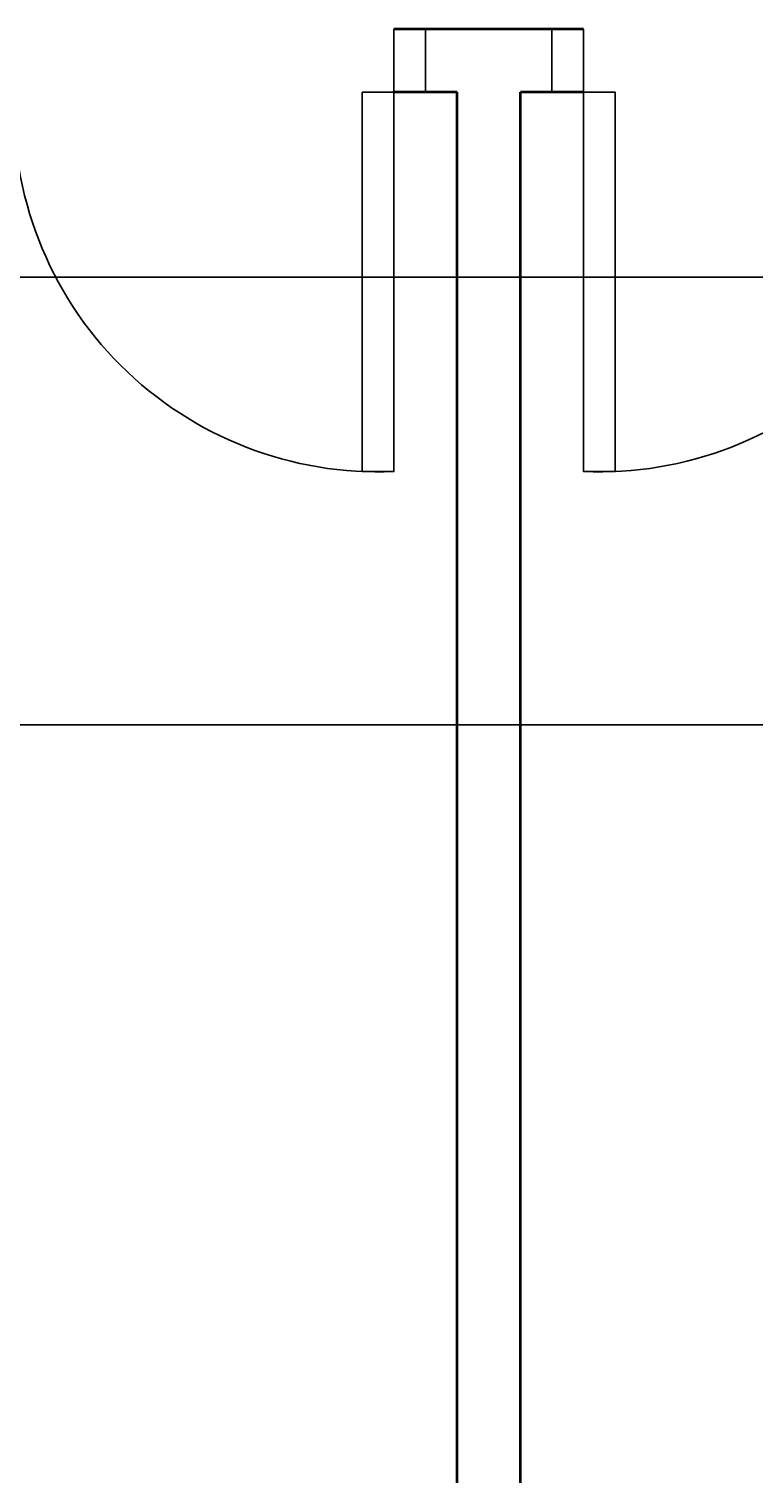
# Model space of a CAD drawing. Units: inches. Extents: x 4159 to 4826, y 299 to 1026.
# Tile 32 of 37: x 4617 to 4685, y 401 to 539. Entities that reach past the tile are written whole.
import ezdxf

# ---------------------------------------------------------------- set-up
doc = ezdxf.new("R2010")
doc.units = ezdxf.units.IN
for name, color, linetype, lineweight in [('A-ANNO-DIMS', 2, 'Continuous', 18), ('A-DOOR', 4, 'Continuous', 25), ('A-WALL', 7, 'Continuous', 35)]:
    doc.layers.add(name, color=color, linetype=linetype, lineweight=lineweight)
doc.styles.get("Standard").update_dxf_attribs({"font": 'arial.ttf'})
doc.dimstyles.get("Standard").update_dxf_attribs({"dimtxt": 0.18, "dimasz": 0.18, "dimexe": 0.18, "dimexo": 0.0625, "dimgap": 0.09, "dimtad": 0, "dimtih": 1, "dimtoh": 1, "dimdec": 4, "dimzin": 0, "dimdsep": 46, "dimtxsty": 'Standard', "dimcen": 0.09, "dimadec": 0, "dimazin": 0, "dimtfac": 1, "dimtdec": 4, "dimtofl": 0, "dimtmove": 0, "dimatfit": 3, "dimfxl": 1, "dimtolj": 1, "dimtzin": 0, "dimarcsym": 0})

# ---------------------------------------------------------------- blocks, each defined once
blk = doc.blocks.new('DOOR-SWING-36IN')
blk.add_lwpolyline([(0, 0), (-3, 0), (-3, 36), (0, 36)], close=True)
blk.add_arc((-1.5, 1.5), 34.53, 87.5104, 182.4896)
blk = doc.blocks.new('DOOR-FRAME-36IN')
for p, q in [((0, 6), (0, 0)), ((3, 6), (3, 0)), ((39, 6), (39, 0)), ((42, 6), (42, 0))]:
    blk.add_line(p, q)
blk = doc.blocks.new('*D54')
at = {"layer": 'A-ANNO-DIMS', "color": 0, "lineweight": -2, "transparency": 16777216}
for p, q in [((4501.37, 515.71), (4825.74, 515.71)), ((4825.56, 515.53), (4825.56, 494.64)), ((4825.56, 473.38), (4825.56, 494.27)), ((4541.95, 473.2), (4825.74, 473.2))]:
    blk.add_line(p, q, dxfattribs=at)
at = {"layer": 'A-ANNO-DIMS', "color": 0, "transparency": 16777216}
for points in [[(4825.53, 515.53), (4825.59, 515.53), (4825.56, 515.71)], [(4825.53, 473.38), (4825.59, 473.38), (4825.56, 473.2)]]:
    blk.add_solid(points, dxfattribs=at)
at = {"layer": 'Defpoints', "color": 0, "transparency": 16777216}
for p in [(4501.31, 515.71), (4825.56, 515.71), (4541.89, 473.2)]:
    blk.add_point(p, dxfattribs=at)
at = {"layer": 'A-ANNO-DIMS', "color": 0, "transparency": 16777216, "insert": (4825.56, 494.45), "char_height": 0.18, "attachment_point": 5}
blk.add_mtext('\\A1;42.52', dxfattribs=at)

msp = doc.modelspace()

# ---------------------------------------------------------------- linework, layer by layer
at = {"layer": 'A-WALL'}
for p, q in [((4669.31, 539.254), (4651.31, 539.254)), ((4657.31, 533.254), (4651.31, 533.254)), ((4657.31, 533.254), (4651.31, 533.254)), ((4657.31, 401.254), (4657.31, 533.254)), ((4663.31, 401.254), (4663.31, 533.254)), ((4669.31, 533.254), (4663.31, 533.254)), ((4669.31, 533.254), (4663.31, 533.254))]:
    msp.add_line(p, q, dxfattribs=at)

# ---------------------------------------------------------------- block references
at = {"layer": 'A-DOOR'}
msp.add_blockref('DOOR-FRAME-36IN', (4612.31, 533.254), dxfattribs=at)
at = {"layer": 'A-DOOR', "rotation": 180}
for name, p in [('DOOR-FRAME-36IN', (4708.31, 539.254)), ('DOOR-SWING-36IN', (4669.31, 533.254))]:
    msp.add_blockref(name, p, dxfattribs=at)
at = {"layer": 'A-DOOR', "extrusion": (0, 0, -1), "zscale": -1, "rotation": 180}
msp.add_blockref('DOOR-SWING-36IN', (-4651.31, 533.254), dxfattribs=at)

# ---------------------------------------------------------------- dimensions: what is measured, and where the dimension line sits
at = {"layer": 'A-ANNO-DIMS'}
dim = msp.add_linear_dim(base=(4825.56, 515.713), p1=(4541.889, 473.195), p2=(4501.31, 515.713), angle=90, dimstyle='Standard', override={"dimdec": 2, "dimlfac": 1, "dimrnd": 0, "dimzin": 0, "dimdsep": 46, "dimlunit": 2}, dxfattribs=at)
dim.commit()
dim.dimension.update_dxf_attribs({"geometry": '*D54', "text_midpoint": (4825.56, 494.454)})

doc.saveas('drawing.dxf')
